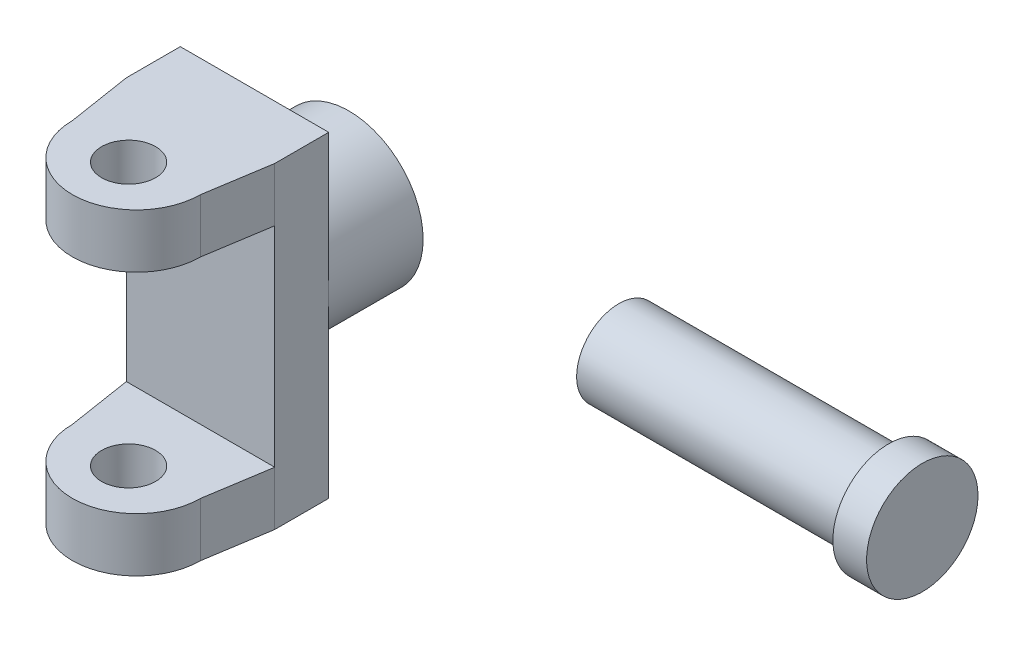
ISO-10303-21;
HEADER;
FILE_DESCRIPTION(('STEP AP214'),'2;1');
FILE_NAME('part.step','',(''),(''),'','','');
FILE_SCHEMA(('AUTOMOTIVE_DESIGN { 1 0 10303 214 1 1 1 1 }'));
ENDSEC;
DATA;
#1=APPLICATION_CONTEXT('core data for automotive mechanical design processes');
#2=APPLICATION_PROTOCOL_DEFINITION('international standard','automotive_design',2000,#1);
#3=PRODUCT_CONTEXT('',#1,'mechanical');
#4=PRODUCT('Part','Part','',(#3));
#5=PRODUCT_RELATED_PRODUCT_CATEGORY('part','',(#4));
#6=PRODUCT_DEFINITION_FORMATION('','',#4);
#7=PRODUCT_DEFINITION_CONTEXT('part definition',#1,'design');
#8=PRODUCT_DEFINITION('design','',#6,#7);
#9=PRODUCT_DEFINITION_SHAPE('','',#8);
#10=(LENGTH_UNIT() NAMED_UNIT(*) SI_UNIT(.MILLI.,.METRE.));
#11=(NAMED_UNIT(*) PLANE_ANGLE_UNIT() SI_UNIT($,.RADIAN.));
#12=(NAMED_UNIT(*) SI_UNIT($,.STERADIAN.) SOLID_ANGLE_UNIT());
#13=UNCERTAINTY_MEASURE_WITH_UNIT(LENGTH_MEASURE(1.E-05),#10,'distance_accuracy_value','');
#14=(GEOMETRIC_REPRESENTATION_CONTEXT(3) GLOBAL_UNCERTAINTY_ASSIGNED_CONTEXT((#13)) GLOBAL_UNIT_ASSIGNED_CONTEXT((#10,
#11,#12)) REPRESENTATION_CONTEXT('',''));
#15=CARTESIAN_POINT('',(0.,0.,0.));
#16=DIRECTION('',(0.,0.,1.));
#17=DIRECTION('',(1.,0.,0.));
#18=AXIS2_PLACEMENT_3D('',#15,#16,#17);
#19=CARTESIAN_POINT('',(340.,0.,0.));
#20=DIRECTION('',(-1.,0.,0.));
#21=DIRECTION('',(0.,0.,1.));
#22=AXIS2_PLACEMENT_3D('',#19,#20,#21);
#23=CYLINDRICAL_SURFACE('',#22,25.);
#24=CARTESIAN_POINT('',(160.,0.,0.));
#25=DIRECTION('',(1.,0.,0.));
#26=DIRECTION('',(0.,0.,-1.));
#27=AXIS2_PLACEMENT_3D('',#24,#25,#26);
#28=CIRCLE('',#27,25.);
#29=CARTESIAN_POINT('',(160.,0.,25.));
#30=VERTEX_POINT('',#29);
#31=EDGE_CURVE('E52',#30,#30,#28,.T.);
#32=CARTESIAN_POINT('',(320.,0.,0.));
#33=DIRECTION('',(1.,0.,0.));
#34=DIRECTION('',(0.,0.,-1.));
#35=AXIS2_PLACEMENT_3D('',#32,#33,#34);
#36=CIRCLE('',#35,25.);
#37=CARTESIAN_POINT('',(320.,0.,25.));
#38=VERTEX_POINT('',#37);
#39=EDGE_CURVE('E11',#38,#38,#36,.T.);
#40=CARTESIAN_POINT('',(160.,0.,25.));
#41=CARTESIAN_POINT('',(161.666666666667,0.,25.));
#42=CARTESIAN_POINT('',(163.333333333333,0.,25.));
#43=CARTESIAN_POINT('',(166.666666666667,0.,25.));
#44=CARTESIAN_POINT('',(168.333333333333,0.,25.));
#45=CARTESIAN_POINT('',(171.666666666667,0.,25.));
#46=CARTESIAN_POINT('',(173.333333333333,0.,25.));
#47=CARTESIAN_POINT('',(176.666666666667,0.,25.));
#48=CARTESIAN_POINT('',(178.333333333333,0.,25.));
#49=CARTESIAN_POINT('',(181.666666666667,0.,25.));
#50=CARTESIAN_POINT('',(183.333333333333,0.,25.));
#51=CARTESIAN_POINT('',(186.666666666667,0.,25.));
#52=CARTESIAN_POINT('',(188.333333333333,0.,25.));
#53=CARTESIAN_POINT('',(191.666666666667,0.,25.));
#54=CARTESIAN_POINT('',(193.333333333333,0.,25.));
#55=CARTESIAN_POINT('',(196.666666666667,0.,25.));
#56=CARTESIAN_POINT('',(198.333333333333,0.,25.));
#57=CARTESIAN_POINT('',(201.666666666667,0.,25.));
#58=CARTESIAN_POINT('',(203.333333333333,0.,25.));
#59=CARTESIAN_POINT('',(206.666666666667,0.,25.));
#60=CARTESIAN_POINT('',(208.333333333333,0.,25.));
#61=CARTESIAN_POINT('',(211.666666666667,0.,25.));
#62=CARTESIAN_POINT('',(213.333333333333,0.,25.));
#63=CARTESIAN_POINT('',(216.666666666667,0.,25.));
#64=CARTESIAN_POINT('',(218.333333333333,0.,25.));
#65=CARTESIAN_POINT('',(221.666666666667,0.,25.));
#66=CARTESIAN_POINT('',(223.333333333333,0.,25.));
#67=CARTESIAN_POINT('',(226.666666666667,0.,25.));
#68=CARTESIAN_POINT('',(228.333333333333,0.,25.));
#69=CARTESIAN_POINT('',(231.666666666667,0.,25.));
#70=CARTESIAN_POINT('',(233.333333333333,0.,25.));
#71=CARTESIAN_POINT('',(236.666666666667,0.,25.));
#72=CARTESIAN_POINT('',(238.333333333333,0.,25.));
#73=CARTESIAN_POINT('',(241.666666666667,0.,25.));
#74=CARTESIAN_POINT('',(243.333333333333,0.,25.));
#75=CARTESIAN_POINT('',(246.666666666667,0.,25.));
#76=CARTESIAN_POINT('',(248.333333333333,0.,25.));
#77=CARTESIAN_POINT('',(251.666666666667,0.,25.));
#78=CARTESIAN_POINT('',(253.333333333333,0.,25.));
#79=CARTESIAN_POINT('',(256.666666666667,0.,25.));
#80=CARTESIAN_POINT('',(258.333333333333,0.,25.));
#81=CARTESIAN_POINT('',(261.666666666667,0.,25.));
#82=CARTESIAN_POINT('',(263.333333333333,0.,25.));
#83=CARTESIAN_POINT('',(266.666666666667,0.,25.));
#84=CARTESIAN_POINT('',(268.333333333333,0.,25.));
#85=CARTESIAN_POINT('',(271.666666666667,0.,25.));
#86=CARTESIAN_POINT('',(273.333333333333,0.,25.));
#87=CARTESIAN_POINT('',(276.666666666667,0.,25.));
#88=CARTESIAN_POINT('',(278.333333333333,0.,25.));
#89=CARTESIAN_POINT('',(281.666666666667,0.,25.));
#90=CARTESIAN_POINT('',(283.333333333333,0.,25.));
#91=CARTESIAN_POINT('',(286.666666666667,0.,25.));
#92=CARTESIAN_POINT('',(288.333333333333,0.,25.));
#93=CARTESIAN_POINT('',(291.666666666667,0.,25.));
#94=CARTESIAN_POINT('',(293.333333333333,0.,25.));
#95=CARTESIAN_POINT('',(296.666666666667,0.,25.));
#96=CARTESIAN_POINT('',(298.333333333333,0.,25.));
#97=CARTESIAN_POINT('',(301.666666666667,0.,25.));
#98=CARTESIAN_POINT('',(303.333333333333,0.,25.));
#99=CARTESIAN_POINT('',(306.666666666667,0.,25.));
#100=CARTESIAN_POINT('',(308.333333333333,0.,25.));
#101=CARTESIAN_POINT('',(311.666666666667,0.,25.));
#102=CARTESIAN_POINT('',(313.333333333333,0.,25.));
#103=CARTESIAN_POINT('',(316.666666666667,0.,25.));
#104=CARTESIAN_POINT('',(318.333333333333,0.,25.));
#105=CARTESIAN_POINT('',(320.,0.,25.));
#106=B_SPLINE_CURVE_WITH_KNOTS('',3,(#40,#41,#42,#43,#44,#45,#46,#47,#48,#49,#50,#51,#52,#53,
#54,#55,#56,#57,#58,#59,#60,#61,#62,#63,#64,#65,#66,#67,#68,#69,#70,#71,#72,#73,#74,#75,#76,#77,
#78,#79,#80,#81,#82,#83,#84,#85,#86,#87,#88,#89,#90,#91,#92,#93,#94,#95,#96,#97,#98,#99,#100,
#101,#102,#103,#104,#105),.UNSPECIFIED.,.F.,.F.,(4,2,2,2,2,2,2,2,2,2,2,2,2,2,2,2,2,2,2,2,2,2,2,
2,2,2,2,2,2,2,2,2,4),(0.,5.,10.,15.,20.,25.,30.,35.,40.,45.,50.,55.,60.,65.,70.,75.,80.,85.,
89.9999999999999,94.9999999999999,99.9999999999999,105.,110.,115.,120.,125.,130.,135.,140.,145.,
150.,155.,160.),.UNSPECIFIED.);
#107=EDGE_CURVE('BSEAM50',#30,#38,#106,.T.);
#108=ORIENTED_EDGE('',*,*,#31,.T.);
#109=ORIENTED_EDGE('',*,*,#39,.F.);
#110=ORIENTED_EDGE('',*,*,#107,.T.);
#111=ORIENTED_EDGE('',*,*,#107,.F.);
#112=EDGE_LOOP('',(#108,#110,#109,#111));
#113=FACE_BOUND('',#112,.T.);
#114=ADVANCED_FACE('F50',(#113),#23,.T.);
#115=CARTESIAN_POINT('',(160.,0.,0.));
#116=DIRECTION('',(1.,0.,0.));
#117=DIRECTION('',(0.,0.,-1.));
#118=AXIS2_PLACEMENT_3D('',#115,#116,#117);
#119=PLANE('',#118);
#120=ORIENTED_EDGE('',*,*,#31,.F.);
#121=EDGE_LOOP('',(#120));
#122=FACE_BOUND('',#121,.T.);
#123=ADVANCED_FACE('F75',(#122),#119,.F.);
#124=CARTESIAN_POINT('',(320.,0.,0.));
#125=DIRECTION('',(1.,0.,0.));
#126=DIRECTION('',(0.,0.,-1.));
#127=AXIS2_PLACEMENT_3D('',#124,#125,#126);
#128=CYLINDRICAL_SURFACE('',#127,33.0290923338109);
#129=CARTESIAN_POINT('',(320.,0.,0.));
#130=DIRECTION('',(1.,0.,0.));
#131=DIRECTION('',(0.,0.,-1.));
#132=AXIS2_PLACEMENT_3D('',#129,#130,#131);
#133=CIRCLE('',#132,33.0290923338109);
#134=CARTESIAN_POINT('',(320.,0.,-33.0290923338109));
#135=VERTEX_POINT('',#134);
#136=EDGE_CURVE('E60',#135,#135,#133,.T.);
#137=ORIENTED_EDGE('',*,*,#136,.T.);
#138=EDGE_LOOP('',(#137));
#139=FACE_BOUND('',#138,.T.);
#140=CARTESIAN_POINT('',(340.,0.,0.));
#141=DIRECTION('',(1.,0.,0.));
#142=DIRECTION('',(0.,0.,-1.));
#143=AXIS2_PLACEMENT_3D('',#140,#141,#142);
#144=CIRCLE('',#143,33.0290923338109);
#145=CARTESIAN_POINT('',(340.,0.,-33.0290923338109));
#146=VERTEX_POINT('',#145);
#147=EDGE_CURVE('E62',#146,#146,#144,.T.);
#148=ORIENTED_EDGE('',*,*,#147,.F.);
#149=EDGE_LOOP('',(#148));
#150=FACE_BOUND('',#149,.T.);
#151=ADVANCED_FACE('F68',(#139,#150),#128,.T.);
#152=CARTESIAN_POINT('',(320.,0.,0.));
#153=DIRECTION('',(1.,0.,0.));
#154=DIRECTION('',(0.,0.,-1.));
#155=AXIS2_PLACEMENT_3D('',#152,#153,#154);
#156=PLANE('',#155);
#157=ORIENTED_EDGE('',*,*,#39,.T.);
#158=EDGE_LOOP('',(#157));
#159=FACE_BOUND('',#158,.T.);
#160=ORIENTED_EDGE('',*,*,#136,.F.);
#161=EDGE_LOOP('',(#160));
#162=FACE_BOUND('',#161,.T.);
#163=ADVANCED_FACE('F72',(#159,#162),#156,.F.);
#164=CARTESIAN_POINT('',(340.,0.,0.));
#165=DIRECTION('',(1.,0.,0.));
#166=DIRECTION('',(0.,0.,-1.));
#167=AXIS2_PLACEMENT_3D('',#164,#165,#166);
#168=PLANE('',#167);
#169=ORIENTED_EDGE('',*,*,#147,.T.);
#170=EDGE_LOOP('',(#169));
#171=FACE_BOUND('',#170,.T.);
#172=ADVANCED_FACE('F66',(#171),#168,.T.);
#173=CLOSED_SHELL('',(#114,#123,#151,#163,#172));
#174=MANIFOLD_SOLID_BREP('B2',#173);
#175=CARTESIAN_POINT('',(0.,0.,88.));
#176=DIRECTION('',(0.,0.,-1.));
#177=DIRECTION('',(-1.,0.,0.));
#178=AXIS2_PLACEMENT_3D('',#175,#176,#177);
#179=PLANE('',#178);
#180=DIRECTION('',(1.,0.,0.));
#181=VECTOR('',#180,1.);
#182=CARTESIAN_POINT('',(-44.,-73.,88.));
#183=LINE('',#182,#181);
#184=CARTESIAN_POINT('',(-44.,-73.,88.));
#185=VERTEX_POINT('',#184);
#186=CARTESIAN_POINT('',(44.,-73.,88.));
#187=VERTEX_POINT('',#186);
#188=EDGE_CURVE('E143',#185,#187,#183,.T.);
#189=ORIENTED_EDGE('',*,*,#188,.T.);
#190=DIRECTION('',(0.,1.,0.));
#191=VECTOR('',#190,1.);
#192=CARTESIAN_POINT('',(44.,83.,88.));
#193=LINE('',#192,#191);
#194=CARTESIAN_POINT('',(44.,51.,88.));
#195=VERTEX_POINT('',#194);
#196=EDGE_CURVE('E302',#187,#195,#193,.T.);
#197=ORIENTED_EDGE('',*,*,#196,.T.);
#198=DIRECTION('',(-1.,0.,0.));
#199=VECTOR('',#198,1.);
#200=CARTESIAN_POINT('',(-44.,51.,88.));
#201=LINE('',#200,#199);
#202=CARTESIAN_POINT('',(-44.,51.,88.));
#203=VERTEX_POINT('',#202);
#204=EDGE_CURVE('E280',#195,#203,#201,.T.);
#205=ORIENTED_EDGE('',*,*,#204,.T.);
#206=DIRECTION('',(0.,-1.,0.));
#207=VECTOR('',#206,1.);
#208=CARTESIAN_POINT('',(-44.,-105.,88.));
#209=LINE('',#208,#207);
#210=EDGE_CURVE('E304',#203,#185,#209,.T.);
#211=ORIENTED_EDGE('',*,*,#210,.T.);
#212=EDGE_LOOP('',(#189,#197,#205,#211));
#213=FACE_BOUND('',#212,.T.);
#214=ADVANCED_FACE('F122',(#213),#179,.F.);
#215=CARTESIAN_POINT('',(0.,0.,56.));
#216=DIRECTION('',(0.,0.,-1.));
#217=DIRECTION('',(-1.,0.,0.));
#218=AXIS2_PLACEMENT_3D('',#215,#216,#217);
#219=CYLINDRICAL_SURFACE('',#218,44.);
#220=CARTESIAN_POINT('',(0.,0.,56.));
#221=DIRECTION('',(0.,0.,1.));
#222=DIRECTION('',(1.,0.,0.));
#223=AXIS2_PLACEMENT_3D('',#220,#221,#222);
#224=CIRCLE('',#223,44.);
#225=CARTESIAN_POINT('',(44.,0.,56.));
#226=VERTEX_POINT('',#225);
#227=CARTESIAN_POINT('',(-44.,0.,56.));
#228=VERTEX_POINT('',#227);
#229=EDGE_CURVE('E44',#226,#228,#224,.T.);
#230=ORIENTED_EDGE('',*,*,#229,.F.);
#231=EDGE_CURVE('E128',#228,#226,#224,.T.);
#232=ORIENTED_EDGE('',*,*,#231,.F.);
#233=EDGE_LOOP('',(#230,#232));
#234=FACE_BOUND('',#233,.T.);
#235=CARTESIAN_POINT('',(0.,0.,0.));
#236=DIRECTION('',(0.,0.,1.));
#237=DIRECTION('',(1.,0.,0.));
#238=AXIS2_PLACEMENT_3D('',#235,#236,#237);
#239=CIRCLE('',#238,44.);
#240=CARTESIAN_POINT('',(44.,0.,0.));
#241=VERTEX_POINT('',#240);
#242=EDGE_CURVE('E364',#241,#241,#239,.T.);
#243=ORIENTED_EDGE('',*,*,#242,.T.);
#244=EDGE_LOOP('',(#243));
#245=FACE_BOUND('',#244,.T.);
#246=ADVANCED_FACE('F124',(#234,#245),#219,.T.);
#247=CARTESIAN_POINT('',(0.,0.,0.));
#248=DIRECTION('',(0.,0.,1.));
#249=DIRECTION('',(1.,0.,0.));
#250=AXIS2_PLACEMENT_3D('',#247,#248,#249);
#251=PLANE('',#250);
#252=DIRECTION('',(0.,-1.,0.));
#253=VECTOR('',#252,1.);
#254=CARTESIAN_POINT('',(-24.98,-0.999799979995997,0.));
#255=LINE('',#254,#253);
#256=CARTESIAN_POINT('',(-24.98,-0.999799979995997,0.));
#257=VERTEX_POINT('',#256);
#258=CARTESIAN_POINT('',(-24.98,-1.000200020004,0.));
#259=VERTEX_POINT('',#258);
#260=EDGE_CURVE('E352',#257,#259,#255,.T.);
#261=ORIENTED_EDGE('',*,*,#260,.F.);
#262=CARTESIAN_POINT('',(0.,0.,0.));
#263=DIRECTION('',(0.,0.,-1.));
#264=DIRECTION('',(-1.,0.,0.));
#265=AXIS2_PLACEMENT_3D('',#262,#263,#264);
#266=CIRCLE('',#265,25.);
#267=CARTESIAN_POINT('',(-24.98,0.999799979996,0.));
#268=VERTEX_POINT('',#267);
#269=EDGE_CURVE('E335',#268,#257,#266,.T.);
#270=ORIENTED_EDGE('',*,*,#269,.F.);
#271=DIRECTION('',(1.,0.,0.));
#272=VECTOR('',#271,1.);
#273=CARTESIAN_POINT('',(-28.2827729461983,0.999799979996,0.));
#274=LINE('',#273,#272);
#275=CARTESIAN_POINT('',(-28.2827729461983,0.999799979996,0.));
#276=VERTEX_POINT('',#275);
#277=EDGE_CURVE('E340',#276,#268,#274,.T.);
#278=ORIENTED_EDGE('',*,*,#277,.F.);
#279=DIRECTION('',(0.,1.,0.));
#280=VECTOR('',#279,1.);
#281=CARTESIAN_POINT('',(-28.2827729461983,-1.000200020004,0.));
#282=LINE('',#281,#280);
#283=CARTESIAN_POINT('',(-28.2827729461983,-1.000200020004,0.));
#284=VERTEX_POINT('',#283);
#285=EDGE_CURVE('E357',#284,#276,#282,.T.);
#286=ORIENTED_EDGE('',*,*,#285,.F.);
#287=DIRECTION('',(-1.,0.,0.));
#288=VECTOR('',#287,1.);
#289=CARTESIAN_POINT('',(-24.98,-1.000200020004,0.));
#290=LINE('',#289,#288);
#291=EDGE_CURVE('E351',#259,#284,#290,.T.);
#292=ORIENTED_EDGE('',*,*,#291,.F.);
#293=EDGE_LOOP('',(#261,#270,#278,#286,#292));
#294=FACE_BOUND('',#293,.T.);
#295=ORIENTED_EDGE('',*,*,#242,.F.);
#296=EDGE_LOOP('',(#295));
#297=FACE_BOUND('',#296,.T.);
#298=ADVANCED_FACE('F422',(#294,#297),#251,.F.);
#299=CARTESIAN_POINT('',(0.,0.,56.));
#300=DIRECTION('',(0.,0.,-1.));
#301=DIRECTION('',(-1.,0.,0.));
#302=AXIS2_PLACEMENT_3D('',#299,#300,#301);
#303=CYLINDRICAL_SURFACE('',#302,25.);
#304=ORIENTED_EDGE('',*,*,#269,.T.);
#305=DIRECTION('',(0.,0.,-1.));
#306=VECTOR('',#305,1.);
#307=CARTESIAN_POINT('',(-24.98,-0.999799979995997,56.));
#308=LINE('',#307,#306);
#309=CARTESIAN_POINT('',(-24.98,-0.999799979995997,56.));
#310=VERTEX_POINT('',#309);
#311=EDGE_CURVE('E348',#310,#257,#308,.T.);
#312=ORIENTED_EDGE('',*,*,#311,.F.);
#313=CARTESIAN_POINT('',(0.,0.,56.));
#314=DIRECTION('',(0.,0.,-1.));
#315=DIRECTION('',(-1.,0.,0.));
#316=AXIS2_PLACEMENT_3D('',#313,#314,#315);
#317=CIRCLE('',#316,25.);
#318=CARTESIAN_POINT('',(-24.98,0.999799979996,56.));
#319=VERTEX_POINT('',#318);
#320=EDGE_CURVE('E334',#319,#310,#317,.T.);
#321=ORIENTED_EDGE('',*,*,#320,.F.);
#322=DIRECTION('',(0.,0.,-1.));
#323=VECTOR('',#322,1.);
#324=CARTESIAN_POINT('',(-24.98,0.999799979996,56.));
#325=LINE('',#324,#323);
#326=EDGE_CURVE('E365',#319,#268,#325,.T.);
#327=ORIENTED_EDGE('',*,*,#326,.T.);
#328=EDGE_LOOP('',(#304,#312,#321,#327));
#329=FACE_BOUND('',#328,.T.);
#330=ADVANCED_FACE('F442',(#329),#303,.F.);
#331=CARTESIAN_POINT('',(-28.2827729461983,0.999799979996,56.));
#332=DIRECTION('',(0.,1.,0.));
#333=DIRECTION('',(-1.,0.,0.));
#334=AXIS2_PLACEMENT_3D('',#331,#332,#333);
#335=PLANE('',#334);
#336=ORIENTED_EDGE('',*,*,#277,.T.);
#337=ORIENTED_EDGE('',*,*,#326,.F.);
#338=DIRECTION('',(1.,0.,0.));
#339=VECTOR('',#338,1.);
#340=CARTESIAN_POINT('',(-28.2827729461983,0.999799979996,56.));
#341=LINE('',#340,#339);
#342=CARTESIAN_POINT('',(-28.2827729461983,0.999799979996,56.));
#343=VERTEX_POINT('',#342);
#344=EDGE_CURVE('E349',#343,#319,#341,.T.);
#345=ORIENTED_EDGE('',*,*,#344,.F.);
#346=DIRECTION('',(0.,0.,-1.));
#347=VECTOR('',#346,1.);
#348=CARTESIAN_POINT('',(-28.2827729461983,0.999799979996,56.));
#349=LINE('',#348,#347);
#350=EDGE_CURVE('E362',#343,#276,#349,.T.);
#351=ORIENTED_EDGE('',*,*,#350,.T.);
#352=EDGE_LOOP('',(#336,#337,#345,#351));
#353=FACE_BOUND('',#352,.T.);
#354=ADVANCED_FACE('F437',(#353),#335,.F.);
#355=CARTESIAN_POINT('',(-28.2827729461983,-1.000200020004,56.));
#356=DIRECTION('',(-1.,0.,0.));
#357=DIRECTION('',(0.,0.,1.));
#358=AXIS2_PLACEMENT_3D('',#355,#356,#357);
#359=PLANE('',#358);
#360=ORIENTED_EDGE('',*,*,#285,.T.);
#361=ORIENTED_EDGE('',*,*,#350,.F.);
#362=DIRECTION('',(0.,1.,0.));
#363=VECTOR('',#362,1.);
#364=CARTESIAN_POINT('',(-28.2827729461983,-1.000200020004,56.));
#365=LINE('',#364,#363);
#366=CARTESIAN_POINT('',(-28.2827729461983,-1.000200020004,56.));
#367=VERTEX_POINT('',#366);
#368=EDGE_CURVE('E344',#367,#343,#365,.T.);
#369=ORIENTED_EDGE('',*,*,#368,.F.);
#370=DIRECTION('',(0.,0.,-1.));
#371=VECTOR('',#370,1.);
#372=CARTESIAN_POINT('',(-28.2827729461983,-1.000200020004,56.));
#373=LINE('',#372,#371);
#374=EDGE_CURVE('E370',#367,#284,#373,.T.);
#375=ORIENTED_EDGE('',*,*,#374,.T.);
#376=EDGE_LOOP('',(#360,#361,#369,#375));
#377=FACE_BOUND('',#376,.T.);
#378=ADVANCED_FACE('F445',(#377),#359,.F.);
#379=CARTESIAN_POINT('',(-24.98,-1.000200020004,56.));
#380=DIRECTION('',(0.,-1.,0.));
#381=DIRECTION('',(0.,0.,-1.));
#382=AXIS2_PLACEMENT_3D('',#379,#380,#381);
#383=PLANE('',#382);
#384=ORIENTED_EDGE('',*,*,#291,.T.);
#385=ORIENTED_EDGE('',*,*,#374,.F.);
#386=DIRECTION('',(-1.,0.,0.));
#387=VECTOR('',#386,1.);
#388=CARTESIAN_POINT('',(-24.98,-1.000200020004,56.));
#389=LINE('',#388,#387);
#390=CARTESIAN_POINT('',(-24.98,-1.000200020004,56.));
#391=VERTEX_POINT('',#390);
#392=EDGE_CURVE('E338',#391,#367,#389,.T.);
#393=ORIENTED_EDGE('',*,*,#392,.F.);
#394=DIRECTION('',(0.,0.,-1.));
#395=VECTOR('',#394,1.);
#396=CARTESIAN_POINT('',(-24.98,-1.000200020004,56.));
#397=LINE('',#396,#395);
#398=EDGE_CURVE('E367',#391,#259,#397,.T.);
#399=ORIENTED_EDGE('',*,*,#398,.T.);
#400=EDGE_LOOP('',(#384,#385,#393,#399));
#401=FACE_BOUND('',#400,.T.);
#402=ADVANCED_FACE('F450',(#401),#383,.F.);
#403=CARTESIAN_POINT('',(-24.98,-0.999799979995997,56.));
#404=DIRECTION('',(1.,0.,0.));
#405=DIRECTION('',(0.,0.,-1.));
#406=AXIS2_PLACEMENT_3D('',#403,#404,#405);
#407=PLANE('',#406);
#408=ORIENTED_EDGE('',*,*,#260,.T.);
#409=ORIENTED_EDGE('',*,*,#398,.F.);
#410=DIRECTION('',(0.,-1.,0.));
#411=VECTOR('',#410,1.);
#412=CARTESIAN_POINT('',(-24.98,-0.999799979995997,56.));
#413=LINE('',#412,#411);
#414=EDGE_CURVE('E337',#310,#391,#413,.T.);
#415=ORIENTED_EDGE('',*,*,#414,.F.);
#416=ORIENTED_EDGE('',*,*,#311,.T.);
#417=EDGE_LOOP('',(#408,#409,#415,#416));
#418=FACE_BOUND('',#417,.T.);
#419=ADVANCED_FACE('F426',(#418),#407,.F.);
#420=CARTESIAN_POINT('',(0.,0.,56.));
#421=DIRECTION('',(0.,0.,-1.));
#422=DIRECTION('',(-1.,0.,0.));
#423=AXIS2_PLACEMENT_3D('',#420,#421,#422);
#424=PLANE('',#423);
#425=DIRECTION('',(0.,-1.,0.));
#426=VECTOR('',#425,1.);
#427=CARTESIAN_POINT('',(-44.,0.,56.));
#428=LINE('',#427,#426);
#429=CARTESIAN_POINT('',(-44.,-105.,56.));
#430=VERTEX_POINT('',#429);
#431=EDGE_CURVE('E320',#228,#430,#428,.T.);
#432=ORIENTED_EDGE('',*,*,#431,.F.);
#433=ORIENTED_EDGE('',*,*,#231,.T.);
#434=DIRECTION('',(0.,1.,0.));
#435=VECTOR('',#434,1.);
#436=CARTESIAN_POINT('',(44.,83.,56.));
#437=LINE('',#436,#435);
#438=CARTESIAN_POINT('',(44.,-105.,56.));
#439=VERTEX_POINT('',#438);
#440=EDGE_CURVE('E315',#439,#226,#437,.T.);
#441=ORIENTED_EDGE('',*,*,#440,.F.);
#442=DIRECTION('',(1.,0.,0.));
#443=VECTOR('',#442,1.);
#444=CARTESIAN_POINT('',(44.,-105.,56.));
#445=LINE('',#444,#443);
#446=EDGE_CURVE('E300',#430,#439,#445,.T.);
#447=ORIENTED_EDGE('',*,*,#446,.F.);
#448=EDGE_LOOP('',(#432,#433,#441,#447));
#449=FACE_BOUND('',#448,.T.);
#450=ADVANCED_FACE('F379',(#449),#424,.T.);
#451=CARTESIAN_POINT('',(-44.,0.,88.));
#452=DIRECTION('',(1.,0.,0.));
#453=DIRECTION('',(0.,0.,-1.));
#454=AXIS2_PLACEMENT_3D('',#451,#452,#453);
#455=PLANE('',#454);
#456=CARTESIAN_POINT('',(-44.,83.,56.));
#457=VERTEX_POINT('',#456);
#458=EDGE_CURVE('E319',#457,#228,#428,.T.);
#459=ORIENTED_EDGE('',*,*,#458,.T.);
#460=ORIENTED_EDGE('',*,*,#431,.T.);
#461=DIRECTION('',(0.,0.,-1.));
#462=VECTOR('',#461,1.);
#463=CARTESIAN_POINT('',(-44.,-105.,88.));
#464=LINE('',#463,#462);
#465=CARTESIAN_POINT('',(-44.,-105.,88.));
#466=VERTEX_POINT('',#465);
#467=EDGE_CURVE('E328',#466,#430,#464,.T.);
#468=ORIENTED_EDGE('',*,*,#467,.F.);
#469=DIRECTION('',(0.,-1.,0.));
#470=VECTOR('',#469,1.);
#471=CARTESIAN_POINT('',(-44.,-73.,88.));
#472=LINE('',#471,#470);
#473=EDGE_CURVE('E139',#185,#466,#472,.T.);
#474=ORIENTED_EDGE('',*,*,#473,.F.);
#475=ORIENTED_EDGE('',*,*,#210,.F.);
#476=CARTESIAN_POINT('',(-44.,83.,88.));
#477=VERTEX_POINT('',#476);
#478=EDGE_CURVE('E301',#477,#203,#209,.T.);
#479=ORIENTED_EDGE('',*,*,#478,.F.);
#480=DIRECTION('',(0.,0.,-1.));
#481=VECTOR('',#480,1.);
#482=CARTESIAN_POINT('',(-44.,83.,88.));
#483=LINE('',#482,#481);
#484=EDGE_CURVE('E307',#477,#457,#483,.T.);
#485=ORIENTED_EDGE('',*,*,#484,.T.);
#486=EDGE_LOOP('',(#459,#460,#468,#474,#475,#479,#485));
#487=FACE_BOUND('',#486,.T.);
#488=ADVANCED_FACE('F397',(#487),#455,.F.);
#489=CARTESIAN_POINT('',(-44.,83.,88.));
#490=DIRECTION('',(0.,-1.,0.));
#491=DIRECTION('',(0.,0.,-1.));
#492=AXIS2_PLACEMENT_3D('',#489,#490,#491);
#493=PLANE('',#492);
#494=CARTESIAN_POINT('',(0.,83.,130.667517763799));
#495=DIRECTION('',(0.,1.,0.));
#496=DIRECTION('',(0.,0.,1.));
#497=AXIS2_PLACEMENT_3D('',#494,#495,#496);
#498=CIRCLE('',#497,16.);
#499=CARTESIAN_POINT('',(0.,83.,146.667517763799));
#500=VERTEX_POINT('',#499);
#501=EDGE_CURVE('E651',#500,#500,#498,.T.);
#502=ORIENTED_EDGE('',*,*,#501,.F.);
#503=EDGE_LOOP('',(#502));
#504=FACE_BOUND('',#503,.T.);
#505=DIRECTION('',(-1.,0.,0.));
#506=VECTOR('',#505,1.);
#507=CARTESIAN_POINT('',(-44.,83.,56.));
#508=LINE('',#507,#506);
#509=CARTESIAN_POINT('',(44.,83.,56.));
#510=VERTEX_POINT('',#509);
#511=EDGE_CURVE('E314',#510,#457,#508,.T.);
#512=ORIENTED_EDGE('',*,*,#511,.T.);
#513=ORIENTED_EDGE('',*,*,#484,.F.);
#514=DIRECTION('',(0.155962573473012,0.,0.987762965329069));
#515=VECTOR('',#514,1.);
#516=CARTESIAN_POINT('',(-44.,83.,88.));
#517=LINE('',#516,#515);
#518=CARTESIAN_POINT('',(-38.,83.,126.));
#519=VERTEX_POINT('',#518);
#520=EDGE_CURVE('E288',#477,#519,#517,.T.);
#521=ORIENTED_EDGE('',*,*,#520,.T.);
#522=CARTESIAN_POINT('',(0.,83.,126.));
#523=DIRECTION('',(0.,1.,0.));
#524=DIRECTION('',(0.,0.,1.));
#525=AXIS2_PLACEMENT_3D('',#522,#523,#524);
#526=CIRCLE('',#525,38.);
#527=CARTESIAN_POINT('',(38.,83.,126.));
#528=VERTEX_POINT('',#527);
#529=EDGE_CURVE('E279',#519,#528,#526,.T.);
#530=ORIENTED_EDGE('',*,*,#529,.T.);
#531=DIRECTION('',(0.155962573473011,0.,-0.987762965329069));
#532=VECTOR('',#531,1.);
#533=CARTESIAN_POINT('',(44.,83.,88.));
#534=LINE('',#533,#532);
#535=CARTESIAN_POINT('',(44.,83.,88.));
#536=VERTEX_POINT('',#535);
#537=EDGE_CURVE('E275',#528,#536,#534,.T.);
#538=ORIENTED_EDGE('',*,*,#537,.T.);
#539=DIRECTION('',(0.,0.,-1.));
#540=VECTOR('',#539,1.);
#541=CARTESIAN_POINT('',(44.,83.,88.));
#542=LINE('',#541,#540);
#543=EDGE_CURVE('E324',#536,#510,#542,.T.);
#544=ORIENTED_EDGE('',*,*,#543,.T.);
#545=EDGE_LOOP('',(#512,#513,#521,#530,#538,#544));
#546=FACE_BOUND('',#545,.T.);
#547=ADVANCED_FACE('F398',(#504,#546),#493,.F.);
#548=CARTESIAN_POINT('',(44.,83.,88.));
#549=DIRECTION('',(-1.,0.,0.));
#550=DIRECTION('',(0.,-1.,0.));
#551=AXIS2_PLACEMENT_3D('',#548,#549,#550);
#552=PLANE('',#551);
#553=ORIENTED_EDGE('',*,*,#440,.T.);
#554=EDGE_CURVE('E311',#226,#510,#437,.T.);
#555=ORIENTED_EDGE('',*,*,#554,.T.);
#556=ORIENTED_EDGE('',*,*,#543,.F.);
#557=DIRECTION('',(0.,1.,0.));
#558=VECTOR('',#557,1.);
#559=CARTESIAN_POINT('',(44.,51.,88.));
#560=LINE('',#559,#558);
#561=EDGE_CURVE('E290',#195,#536,#560,.T.);
#562=ORIENTED_EDGE('',*,*,#561,.F.);
#563=ORIENTED_EDGE('',*,*,#196,.F.);
#564=CARTESIAN_POINT('',(44.,-105.,88.));
#565=VERTEX_POINT('',#564);
#566=EDGE_CURVE('E306',#565,#187,#193,.T.);
#567=ORIENTED_EDGE('',*,*,#566,.F.);
#568=DIRECTION('',(0.,0.,-1.));
#569=VECTOR('',#568,1.);
#570=CARTESIAN_POINT('',(44.,-105.,88.));
#571=LINE('',#570,#569);
#572=EDGE_CURVE('E329',#565,#439,#571,.T.);
#573=ORIENTED_EDGE('',*,*,#572,.T.);
#574=EDGE_LOOP('',(#553,#555,#556,#562,#563,#567,#573));
#575=FACE_BOUND('',#574,.T.);
#576=ADVANCED_FACE('F386',(#575),#552,.F.);
#577=CARTESIAN_POINT('',(44.,-105.,88.));
#578=DIRECTION('',(0.,1.,0.));
#579=DIRECTION('',(0.,0.,1.));
#580=AXIS2_PLACEMENT_3D('',#577,#578,#579);
#581=PLANE('',#580);
#582=CARTESIAN_POINT('',(0.,-105.,130.667517763799));
#583=DIRECTION('',(0.,1.,0.));
#584=DIRECTION('',(0.,0.,1.));
#585=AXIS2_PLACEMENT_3D('',#582,#583,#584);
#586=CIRCLE('',#585,16.);
#587=CARTESIAN_POINT('',(0.,-105.,146.667517763799));
#588=VERTEX_POINT('',#587);
#589=EDGE_CURVE('E265',#588,#588,#586,.T.);
#590=ORIENTED_EDGE('',*,*,#589,.T.);
#591=EDGE_LOOP('',(#590));
#592=FACE_BOUND('',#591,.T.);
#593=ORIENTED_EDGE('',*,*,#446,.T.);
#594=ORIENTED_EDGE('',*,*,#572,.F.);
#595=DIRECTION('',(-0.155962573473011,0.,0.987762965329069));
#596=VECTOR('',#595,1.);
#597=CARTESIAN_POINT('',(44.,-105.,88.));
#598=LINE('',#597,#596);
#599=CARTESIAN_POINT('',(38.,-105.,126.));
#600=VERTEX_POINT('',#599);
#601=EDGE_CURVE('E259',#565,#600,#598,.T.);
#602=ORIENTED_EDGE('',*,*,#601,.T.);
#603=CARTESIAN_POINT('',(0.,-105.,126.));
#604=DIRECTION('',(0.,-1.,0.));
#605=DIRECTION('',(0.,0.,-1.));
#606=AXIS2_PLACEMENT_3D('',#603,#604,#605);
#607=CIRCLE('',#606,38.);
#608=CARTESIAN_POINT('',(-38.,-105.,126.));
#609=VERTEX_POINT('',#608);
#610=EDGE_CURVE('E269',#600,#609,#607,.T.);
#611=ORIENTED_EDGE('',*,*,#610,.T.);
#612=DIRECTION('',(-0.155962573473012,0.,-0.987762965329069));
#613=VECTOR('',#612,1.);
#614=CARTESIAN_POINT('',(-38.,-105.,126.));
#615=LINE('',#614,#613);
#616=EDGE_CURVE('E245',#609,#466,#615,.T.);
#617=ORIENTED_EDGE('',*,*,#616,.T.);
#618=ORIENTED_EDGE('',*,*,#467,.T.);
#619=EDGE_LOOP('',(#593,#594,#602,#611,#617,#618));
#620=FACE_BOUND('',#619,.T.);
#621=ADVANCED_FACE('F395',(#592,#620),#581,.F.);
#622=ORIENTED_EDGE('',*,*,#554,.F.);
#623=ORIENTED_EDGE('',*,*,#229,.T.);
#624=ORIENTED_EDGE('',*,*,#458,.F.);
#625=ORIENTED_EDGE('',*,*,#511,.F.);
#626=EDGE_LOOP('',(#622,#623,#624,#625));
#627=FACE_BOUND('',#626,.T.);
#628=ADVANCED_FACE('F383',(#627),#424,.T.);
#629=ORIENTED_EDGE('',*,*,#344,.T.);
#630=ORIENTED_EDGE('',*,*,#320,.T.);
#631=ORIENTED_EDGE('',*,*,#414,.T.);
#632=ORIENTED_EDGE('',*,*,#392,.T.);
#633=ORIENTED_EDGE('',*,*,#368,.T.);
#634=EDGE_LOOP('',(#629,#630,#631,#632,#633));
#635=FACE_BOUND('',#634,.T.);
#636=ADVANCED_FACE('F429',(#635),#424,.T.);
#637=CARTESIAN_POINT('',(44.,51.,88.));
#638=DIRECTION('',(0.987762965329069,0.,0.155962573473011));
#639=DIRECTION('',(0.155962573473011,0.,-0.987762965329069));
#640=AXIS2_PLACEMENT_3D('',#637,#638,#639);
#641=PLANE('',#640);
#642=ORIENTED_EDGE('',*,*,#537,.F.);
#643=DIRECTION('',(0.,1.,0.));
#644=VECTOR('',#643,1.);
#645=CARTESIAN_POINT('',(38.,51.,126.));
#646=LINE('',#645,#644);
#647=CARTESIAN_POINT('',(38.,51.,126.));
#648=VERTEX_POINT('',#647);
#649=EDGE_CURVE('E294',#648,#528,#646,.T.);
#650=ORIENTED_EDGE('',*,*,#649,.F.);
#651=DIRECTION('',(0.155962573473011,0.,-0.987762965329069));
#652=VECTOR('',#651,1.);
#653=CARTESIAN_POINT('',(44.,51.,88.));
#654=LINE('',#653,#652);
#655=EDGE_CURVE('E274',#648,#195,#654,.T.);
#656=ORIENTED_EDGE('',*,*,#655,.T.);
#657=ORIENTED_EDGE('',*,*,#561,.T.);
#658=EDGE_LOOP('',(#642,#650,#656,#657));
#659=FACE_BOUND('',#658,.T.);
#660=ADVANCED_FACE('F403',(#659),#641,.T.);
#661=CARTESIAN_POINT('',(0.,51.,126.));
#662=DIRECTION('',(0.,1.,0.));
#663=DIRECTION('',(0.,0.,1.));
#664=AXIS2_PLACEMENT_3D('',#661,#662,#663);
#665=CYLINDRICAL_SURFACE('',#664,38.);
#666=ORIENTED_EDGE('',*,*,#529,.F.);
#667=DIRECTION('',(0.,1.,0.));
#668=VECTOR('',#667,1.);
#669=CARTESIAN_POINT('',(-38.,51.,126.));
#670=LINE('',#669,#668);
#671=CARTESIAN_POINT('',(-38.,51.,126.));
#672=VERTEX_POINT('',#671);
#673=EDGE_CURVE('E296',#672,#519,#670,.T.);
#674=ORIENTED_EDGE('',*,*,#673,.F.);
#675=CARTESIAN_POINT('',(0.,51.,126.));
#676=DIRECTION('',(0.,1.,0.));
#677=DIRECTION('',(0.,0.,1.));
#678=AXIS2_PLACEMENT_3D('',#675,#676,#677);
#679=CIRCLE('',#678,38.);
#680=EDGE_CURVE('E283',#672,#648,#679,.T.);
#681=ORIENTED_EDGE('',*,*,#680,.T.);
#682=ORIENTED_EDGE('',*,*,#649,.T.);
#683=EDGE_LOOP('',(#666,#674,#681,#682));
#684=FACE_BOUND('',#683,.T.);
#685=ADVANCED_FACE('F411',(#684),#665,.T.);
#686=CARTESIAN_POINT('',(-44.,51.,88.));
#687=DIRECTION('',(-0.987762965329069,0.,0.155962573473012));
#688=DIRECTION('',(0.155962573473012,0.,0.987762965329069));
#689=AXIS2_PLACEMENT_3D('',#686,#687,#688);
#690=PLANE('',#689);
#691=ORIENTED_EDGE('',*,*,#520,.F.);
#692=ORIENTED_EDGE('',*,*,#478,.T.);
#693=DIRECTION('',(0.155962573473012,0.,0.987762965329069));
#694=VECTOR('',#693,1.);
#695=CARTESIAN_POINT('',(-44.,51.,88.));
#696=LINE('',#695,#694);
#697=EDGE_CURVE('E284',#203,#672,#696,.T.);
#698=ORIENTED_EDGE('',*,*,#697,.T.);
#699=ORIENTED_EDGE('',*,*,#673,.T.);
#700=EDGE_LOOP('',(#691,#692,#698,#699));
#701=FACE_BOUND('',#700,.T.);
#702=ADVANCED_FACE('F413',(#701),#690,.T.);
#703=CARTESIAN_POINT('',(0.,51.,126.));
#704=DIRECTION('',(0.,1.,0.));
#705=DIRECTION('',(0.,0.,1.));
#706=AXIS2_PLACEMENT_3D('',#703,#704,#705);
#707=PLANE('',#706);
#708=CARTESIAN_POINT('',(0.,51.,130.667517763799));
#709=DIRECTION('',(0.,1.,0.));
#710=DIRECTION('',(0.,0.,1.));
#711=AXIS2_PLACEMENT_3D('',#708,#709,#710);
#712=CIRCLE('',#711,16.);
#713=CARTESIAN_POINT('',(0.,51.,146.667517763799));
#714=VERTEX_POINT('',#713);
#715=EDGE_CURVE('E652',#714,#714,#712,.T.);
#716=ORIENTED_EDGE('',*,*,#715,.T.);
#717=EDGE_LOOP('',(#716));
#718=FACE_BOUND('',#717,.T.);
#719=ORIENTED_EDGE('',*,*,#655,.F.);
#720=ORIENTED_EDGE('',*,*,#680,.F.);
#721=ORIENTED_EDGE('',*,*,#697,.F.);
#722=ORIENTED_EDGE('',*,*,#204,.F.);
#723=EDGE_LOOP('',(#719,#720,#721,#722));
#724=FACE_BOUND('',#723,.T.);
#725=ADVANCED_FACE('F408',(#718,#724),#707,.F.);
#726=CARTESIAN_POINT('',(0.,-73.,126.));
#727=DIRECTION('',(0.,-1.,0.));
#728=DIRECTION('',(0.,0.,-1.));
#729=AXIS2_PLACEMENT_3D('',#726,#727,#728);
#730=CYLINDRICAL_SURFACE('',#729,38.);
#731=ORIENTED_EDGE('',*,*,#610,.F.);
#732=DIRECTION('',(0.,-1.,0.));
#733=VECTOR('',#732,1.);
#734=CARTESIAN_POINT('',(38.,-73.,126.));
#735=LINE('',#734,#733);
#736=CARTESIAN_POINT('',(38.,-73.,126.));
#737=VERTEX_POINT('',#736);
#738=EDGE_CURVE('E260',#737,#600,#735,.T.);
#739=ORIENTED_EDGE('',*,*,#738,.F.);
#740=CARTESIAN_POINT('',(0.,-73.,126.));
#741=DIRECTION('',(0.,-1.,0.));
#742=DIRECTION('',(0.,0.,-1.));
#743=AXIS2_PLACEMENT_3D('',#740,#741,#742);
#744=CIRCLE('',#743,38.);
#745=CARTESIAN_POINT('',(-38.,-73.,126.));
#746=VERTEX_POINT('',#745);
#747=EDGE_CURVE('E254',#737,#746,#744,.T.);
#748=ORIENTED_EDGE('',*,*,#747,.T.);
#749=DIRECTION('',(0.,-1.,0.));
#750=VECTOR('',#749,1.);
#751=CARTESIAN_POINT('',(-38.,-73.,126.));
#752=LINE('',#751,#750);
#753=EDGE_CURVE('E240',#746,#609,#752,.T.);
#754=ORIENTED_EDGE('',*,*,#753,.T.);
#755=EDGE_LOOP('',(#731,#739,#748,#754));
#756=FACE_BOUND('',#755,.T.);
#757=ADVANCED_FACE('F257',(#756),#730,.T.);
#758=CARTESIAN_POINT('',(44.,-73.,88.));
#759=DIRECTION('',(0.987762965329069,0.,0.155962573473011));
#760=DIRECTION('',(0.155962573473011,0.,-0.987762965329069));
#761=AXIS2_PLACEMENT_3D('',#758,#759,#760);
#762=PLANE('',#761);
#763=ORIENTED_EDGE('',*,*,#601,.F.);
#764=ORIENTED_EDGE('',*,*,#566,.T.);
#765=DIRECTION('',(-0.155962573473011,0.,0.987762965329069));
#766=VECTOR('',#765,1.);
#767=CARTESIAN_POINT('',(44.,-73.,88.));
#768=LINE('',#767,#766);
#769=EDGE_CURVE('E250',#187,#737,#768,.T.);
#770=ORIENTED_EDGE('',*,*,#769,.T.);
#771=ORIENTED_EDGE('',*,*,#738,.T.);
#772=EDGE_LOOP('',(#763,#764,#770,#771));
#773=FACE_BOUND('',#772,.T.);
#774=ADVANCED_FACE('F392',(#773),#762,.T.);
#775=CARTESIAN_POINT('',(-38.,-73.,126.));
#776=DIRECTION('',(-0.987762965329069,0.,0.155962573473012));
#777=DIRECTION('',(0.155962573473012,0.,0.987762965329069));
#778=AXIS2_PLACEMENT_3D('',#775,#776,#777);
#779=PLANE('',#778);
#780=ORIENTED_EDGE('',*,*,#616,.F.);
#781=ORIENTED_EDGE('',*,*,#753,.F.);
#782=DIRECTION('',(-0.155962573473012,0.,-0.987762965329069));
#783=VECTOR('',#782,1.);
#784=CARTESIAN_POINT('',(-38.,-73.,126.));
#785=LINE('',#784,#783);
#786=EDGE_CURVE('E239',#746,#185,#785,.T.);
#787=ORIENTED_EDGE('',*,*,#786,.T.);
#788=ORIENTED_EDGE('',*,*,#473,.T.);
#789=EDGE_LOOP('',(#780,#781,#787,#788));
#790=FACE_BOUND('',#789,.T.);
#791=ADVANCED_FACE('F237',(#790),#779,.T.);
#792=CARTESIAN_POINT('',(0.,-73.,126.));
#793=DIRECTION('',(0.,-1.,0.));
#794=DIRECTION('',(0.,0.,-1.));
#795=AXIS2_PLACEMENT_3D('',#792,#793,#794);
#796=PLANE('',#795);
#797=CARTESIAN_POINT('',(0.,-73.,130.667517763799));
#798=DIRECTION('',(0.,-1.,0.));
#799=DIRECTION('',(0.,0.,-1.));
#800=AXIS2_PLACEMENT_3D('',#797,#798,#799);
#801=CIRCLE('',#800,16.);
#802=CARTESIAN_POINT('',(0.,-73.,114.667517763799));
#803=VERTEX_POINT('',#802);
#804=EDGE_CURVE('E123',#803,#803,#801,.T.);
#805=ORIENTED_EDGE('',*,*,#804,.T.);
#806=EDGE_LOOP('',(#805));
#807=FACE_BOUND('',#806,.T.);
#808=ORIENTED_EDGE('',*,*,#747,.F.);
#809=ORIENTED_EDGE('',*,*,#769,.F.);
#810=ORIENTED_EDGE('',*,*,#188,.F.);
#811=ORIENTED_EDGE('',*,*,#786,.F.);
#812=EDGE_LOOP('',(#808,#809,#810,#811));
#813=FACE_BOUND('',#812,.T.);
#814=ADVANCED_FACE('F252',(#807,#813),#796,.F.);
#815=CARTESIAN_POINT('',(0.,-615.,130.667517763799));
#816=DIRECTION('',(0.,1.,0.));
#817=DIRECTION('',(0.,0.,1.));
#818=AXIS2_PLACEMENT_3D('',#815,#816,#817);
#819=CYLINDRICAL_SURFACE('',#818,16.);
#820=ORIENTED_EDGE('',*,*,#804,.F.);
#821=EDGE_LOOP('',(#820));
#822=FACE_BOUND('',#821,.T.);
#823=ORIENTED_EDGE('',*,*,#589,.F.);
#824=EDGE_LOOP('',(#823));
#825=FACE_BOUND('',#824,.T.);
#826=ADVANCED_FACE('F615',(#822,#825),#819,.F.);
#827=ORIENTED_EDGE('',*,*,#501,.T.);
#828=EDGE_LOOP('',(#827));
#829=FACE_BOUND('',#828,.T.);
#830=ORIENTED_EDGE('',*,*,#715,.F.);
#831=EDGE_LOOP('',(#830));
#832=FACE_BOUND('',#831,.T.);
#833=ADVANCED_FACE('F623',(#829,#832),#819,.F.);
#834=CLOSED_SHELL('',(#214,#246,#298,#330,#354,#378,#402,#419,#450,#488,#547,#576,#621,#628,
#636,#660,#685,#702,#725,#757,#774,#791,#814,#826,#833));
#835=MANIFOLD_SOLID_BREP('B6',#834);
#836=ADVANCED_BREP_SHAPE_REPRESENTATION('',(#18,#174,#835),#14);
#837=SHAPE_DEFINITION_REPRESENTATION(#9,#836);
ENDSEC;
END-ISO-10303-21;
